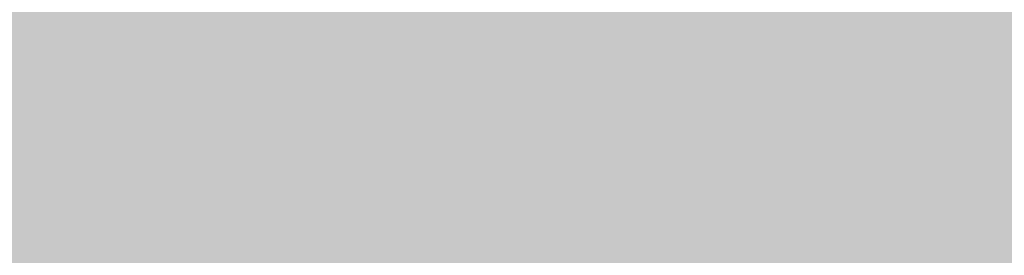
# Model space of a CAD drawing. Units: millimetres. Extents: x 0 to 2267, y 0 to 1823.
# Tile 200 of 256: x 1838.83 to 1841.442, y 1127.775 to 1128.399. Entities that reach past the tile are written whole.
import ezdxf

# ---------------------------------------------------------------- set-up
doc = ezdxf.new("R2010")
doc.units = ezdxf.units.MM
doc.header["$MEASUREMENT"] = 0
doc.layers.add('M-HATC', color=252, linetype='Continuous', lineweight=18)

msp = doc.modelspace()

# ---------------------------------------------------------------- hatches: boundary and pattern name
at = {"layer": 'M-HATC'}
h = msp.add_hatch(color=256, dxfattribs=at)
h.dxf.hatch_style = 1
h.paths.add_polyline_path([(2055.771, 1603.062), (1381.0868, 1603.062), (1381.0868, 1598.062), (2055.771, 1598.062)])
h.paths.add_polyline_path([(2055.771, 1598.062), (1381.0868, 1598.062), (1381.0868, 1593.062), (2055.771, 1593.062)])
h.paths.add_polyline_path([(2051.3074, 1536.7609), (1385.5504, 1536.7609), (1385.5504, 1526.7609), (1387.5504, 1526.7609), (1388.5366, 1525.0528), (1385.3319, 1521.2335), (1385.3319, 1521.2226), (2050.2542, 1522.7491), (2048.3212, 1525.0528), (2049.3074, 1526.7609), (2051.3074, 1526.7609)])
edge = h.paths.add_edge_path()
edge.add_arc((1847.5345, 1379.1492), 135, 222.603061, 222.890851, ccw=False)
edge.add_line((1748.1663, 1287.7656), (1683.0921, 1287.7656))
edge.add_arc((1583.7239, 1379.1492), 135, 317.109149, 317.396939, ccw=False)
edge.add_arc((1678.9686, 1290.6707), 5, 222.8909, 317.1091, ccw=False)
edge.add_arc((1774.2133, 1379.1492), 135, 222.603061, 222.890851, ccw=False)
edge.add_line((1674.8451, 1287.7656), (1609.7709, 1287.7656))
edge.add_arc((1510.4027, 1379.1492), 135, 317.109149, 317.396939, ccw=False)
edge.add_arc((1605.6474, 1290.6707), 5, 222.8909, 317.1091, ccw=False)
edge.add_arc((1700.8921, 1379.1492), 135, 222.603061, 222.890851, ccw=False)
edge.add_line((1601.5239, 1287.7656), (1536.4497, 1287.7656))
edge.add_arc((1437.0815, 1379.1492), 135, 317.109149, 317.396939, ccw=False)
edge.add_arc((1532.3262, 1290.6707), 5, 222.8909, 317.1091, ccw=False)
edge.add_arc((1627.5709, 1379.1492), 135, 222.603061, 222.890851, ccw=False)
edge.add_line((1528.2027, 1287.7656), (1505.9289, 1287.7656))
edge.add_spline(control_points=[(1505.9289, 1287.7656), (1504.2622, 1287.7656), (1504.2622, 1282.7656), (1505.9289, 1282.7656)], knot_values=[0, 0, 0, 0, 5, 5, 5, 5], degree=3, periodic=0)
edge.add_line((1505.9289, 1282.7656), (1930.9289, 1282.7656))
edge.add_spline(control_points=[(1930.9289, 1282.7656), (1932.5956, 1282.7656), (1932.5956, 1287.7656), (1930.9289, 1287.7656)], knot_values=[0, 0, 0, 0, 5, 5, 5, 5], degree=3, periodic=0)
edge.add_line((1930.9289, 1287.7656), (1903.0557, 1287.7656))
edge.add_arc((1803.6875, 1379.1492), 135, 317.109149, 317.396939, ccw=False)
edge.add_arc((1898.9322, 1290.6707), 5, 222.8909, 317.1091, ccw=False)
edge.add_arc((1994.1769, 1379.1492), 135, 222.603061, 222.890851, ccw=False)
edge.add_line((1894.8087, 1287.7656), (1829.7345, 1287.7656))
edge.add_arc((1730.3663, 1379.1492), 135, 317.109149, 317.396939, ccw=False)
edge.add_arc((1825.611, 1290.6707), 5, 222.8909, 317.1091, ccw=False)
edge.add_arc((1920.8557, 1379.1492), 135, 222.603061, 222.890851, ccw=False)
edge.add_line((1821.4875, 1287.7656), (1756.4133, 1287.7656))
edge.add_arc((1657.0451, 1379.1492), 135, 317.109149, 317.396939, ccw=False)
edge.add_arc((1752.2898, 1290.6707), 5, 222.8909, 317.1091, ccw=False)
edge = h.paths.add_edge_path()
edge.add_spline(control_points=[(1843.4289, 1227.2475), (1845.0956, 1227.2475), (1845.0956, 1232.2475), (1843.4289, 1232.2475)], knot_values=[0, 0, 0, 0, 5, 5, 5, 5], degree=3, periodic=0)
edge.add_line((1843.4289, 1232.2475), (1593.4289, 1232.2475))
edge.add_spline(control_points=[(1593.4289, 1232.2475), (1591.7622, 1232.2475), (1591.7622, 1227.2475), (1593.4289, 1227.2475)], knot_values=[0, 0, 0, 0, 5, 5, 5, 5], degree=3, periodic=0)
edge.add_line((1593.4289, 1227.2475), (1843.4289, 1227.2475))
h.paths.add_polyline_path([(1905.9289, 1127.4171), (1530.9289, 1127.4171, 0.414214), (1520.9289, 1117.4171), (1530.9289, 1117.4171), (1915.9289, 1117.4171, 0.414214)])
edge = h.paths.add_edge_path()
edge.add_arc((1397.0858, 1498.4078), 12.7299, 90.78215, 190.87871, ccw=False)
edge.add_line((1396.912, 1511.1365), (1428.0097, 1511.3488))
edge.add_line((1428.0097, 1511.3488), (1433.0097, 1511.3488))
edge.add_line((1433.0097, 1511.3488), (1434.439, 1511.3488))
edge.add_arc((1419.474, 1498.0804), 20, 41.561, 74.08211)
edge.add_line((1424.9592, 1517.3135), (1399.9351, 1517.2561))
edge.add_spline(control_points=[(1399.9307, 1517.2561), (1399.884, 1517.2131), (1399.8328, 1517.1689), (1399.7774, 1517.1236)], knot_values=[11.567499, 11.567499, 11.567499, 11.567499, 11.814249, 11.814249, 11.814249, 11.814249], degree=3, periodic=0)
edge.add_spline(control_points=[(1399.6328, 1517.0099), (1399.5831, 1516.9721), (1399.5307, 1516.9338), (1399.4759, 1516.8947)], knot_values=[11.167718, 11.167718, 11.167718, 11.167718, 11.365188, 11.365188, 11.365188, 11.365188], degree=3, periodic=0)
edge.add_spline(control_points=[(1399.3398, 1516.8001), (1399.1514, 1516.6719), (1398.9384, 1516.5377), (1398.704, 1516.3994)], knot_values=[10.376405, 10.376405, 10.376405, 10.376405, 11.00994, 11.00994, 11.00994, 11.00994], degree=3, periodic=0)
edge.add_spline(control_points=[(1398.6572, 1516.3719), (1398.5789, 1516.326), (1398.4983, 1516.2797), (1398.4155, 1516.2331)], knot_values=[10.125175, 10.125175, 10.125175, 10.125175, 10.334406, 10.334406, 10.334406, 10.334406], degree=3, periodic=0)
edge.add_spline(control_points=[(1398.2642, 1516.1487), (1398.196, 1516.1111), (1398.1263, 1516.0732), (1398.0555, 1516.0351)], knot_values=[9.832246, 9.832246, 9.832246, 9.832246, 9.999658, 9.999658, 9.999658, 9.999658], degree=3, periodic=0)
edge.add_spline(control_points=[(1397.9987, 1516.0048), (1397.7312, 1515.8621), (1397.446, 1515.7171), (1397.1466, 1515.5714)], knot_values=[9.161808, 9.161808, 9.161808, 9.161808, 9.787769, 9.787769, 9.787769, 9.787769], degree=3, periodic=0)
edge.add_spline(control_points=[(1397.1466, 1515.5714), (1396.8418, 1515.423), (1396.5222, 1515.274), (1396.1914, 1515.1262)], knot_values=[8.524455, 8.524455, 8.524455, 8.524455, 9.161808, 9.161808, 9.161808, 9.161808], degree=3, periodic=0)
edge.add_spline(control_points=[(1396.0777, 1515.0756), (1395.9854, 1515.0348), (1395.8922, 1514.994), (1395.7983, 1514.9534)], knot_values=[8.275193, 8.275193, 8.275193, 8.275193, 8.451726, 8.451726, 8.451726, 8.451726], degree=3, periodic=0)
edge.add_spline(control_points=[(1395.6018, 1514.8691), (1395.4997, 1514.8257), (1395.3968, 1514.7824), (1395.2932, 1514.7394)], knot_values=[7.962917, 7.962917, 7.962917, 7.962917, 8.152764, 8.152764, 8.152764, 8.152764], degree=3, periodic=0)
edge.add_spline(control_points=[(1395.2116, 1514.7057), (1394.8278, 1514.5475), (1394.4345, 1514.3929), (1394.0364, 1514.2442)], knot_values=[7.21254, 7.21254, 7.21254, 7.21254, 7.913148, 7.913148, 7.913148, 7.913148], degree=3, periodic=0)
edge.add_spline(control_points=[(1394.0364, 1514.2442), (1393.7076, 1514.1214), (1393.3754, 1514.0027), (1393.0427, 1513.8895)], knot_values=[6.633733, 6.633733, 6.633733, 6.633733, 7.21254, 7.21254, 7.21254, 7.21254], degree=3, periodic=0)
edge.add_spline(control_points=[(1392.8214, 1513.815), (1392.7198, 1513.7812), (1392.6181, 1513.7479), (1392.5166, 1513.7152)], knot_values=[6.328796, 6.328796, 6.328796, 6.328796, 6.505493, 6.505493, 6.505493, 6.505493], degree=3, periodic=0)
edge.add_spline(control_points=[(1392.5166, 1513.7152), (1392.3187, 1513.6515), (1392.1212, 1513.59), (1391.9244, 1513.531)], knot_values=[5.984605, 5.984605, 5.984605, 5.984605, 6.328796, 6.328796, 6.328796, 6.328796], degree=3, periodic=0)
edge.add_spline(control_points=[(1391.7915, 1513.4915), (1391.3122, 1513.3501), (1390.8384, 1513.2239), (1390.3784, 1513.1171)], knot_values=[5.066697, 5.066697, 5.066697, 5.066697, 5.907055, 5.907055, 5.907055, 5.907055], degree=3, periodic=0)
edge.add_spline(control_points=[(1390.3784, 1513.1171), (1390.1797, 1513.071), (1389.9836, 1513.0284), (1389.7907, 1512.9899)], knot_values=[4.70367, 4.70367, 4.70367, 4.70367, 5.066695, 5.066695, 5.066695, 5.066695], degree=3, periodic=0)
edge.add_spline(control_points=[(1389.422, 1512.9204), (1389.2459, 1512.8892), (1389.0729, 1512.8617), (1388.9036, 1512.8381)], knot_values=[4.130571, 4.130571, 4.130571, 4.130571, 4.469816, 4.469816, 4.469816, 4.469816], degree=3, periodic=0)
edge.add_spline(control_points=[(1388.9036, 1512.8381), (1388.591, 1512.7946), (1388.2911, 1512.7644), (1388.0071, 1512.7494)], knot_values=[3.504031, 3.504031, 3.504031, 3.504031, 4.130571, 4.130571, 4.130571, 4.130571], degree=3, periodic=0)
edge.add_spline(control_points=[(1387.9356, 1512.7459), (1387.8538, 1512.7423), (1387.7733, 1512.74), (1387.6944, 1512.739)], knot_values=[3.268866, 3.268866, 3.268866, 3.268866, 3.451164, 3.451164, 3.451164, 3.451164], degree=3, periodic=0)
edge.add_spline(control_points=[(1387.3351, 1512.7443), (1387.2076, 1512.7499), (1387.0847, 1512.7597), (1386.967, 1512.7739)], knot_values=[2.670686, 2.670686, 2.670686, 2.670686, 2.984, 2.984, 2.984, 2.984], degree=3, periodic=0)
edge.add_spline(control_points=[(1386.8327, 1512.7922), (1386.8209, 1512.7941), (1386.8092, 1512.7959), (1386.7975, 1512.7979)], knot_values=[2.516981, 2.516981, 2.516981, 2.516981, 2.549528, 2.549528, 2.549528, 2.549528], degree=3, periodic=0)
edge.add_spline(control_points=[(1386.4526, 1512.8735), (1386.4257, 1512.881), (1386.3993, 1512.889), (1386.3733, 1512.8972)], knot_values=[2.095869, 2.095869, 2.095869, 2.095869, 2.17941, 2.17941, 2.17941, 2.17941], degree=3, periodic=0)
edge.add_spline(control_points=[(1386.0691, 1513.0189), (1386.0634, 1513.0217), (1386.0577, 1513.0246), (1386.052, 1513.0275)], knot_values=[1.72453, 1.72453, 1.72453, 1.72453, 1.745933, 1.745933, 1.745933, 1.745933], degree=3, periodic=0)
edge.add_arc((1399.474, 1498.0804), 20, 131.82432, 180)
edge.add_arc((1630.3336, 1505.5484), 250.9708, 181.705176, 236.427975)
edge.add_arc((1605.3399, 1483.3044), 218.7822, 238.660829, 243.34961)
edge.add_arc((1647.0911, 1510.3592), 262.8986, 183.129836, 237.853442, ccw=False)
h.paths.add_polyline_path([(1406.5369, 1391.9644, 0.149382), (1491.5506, 1296.4418, -0.129517)], flags=17)
edge = h.paths.add_edge_path()
edge.add_arc((2037.3838, 1498.0804), 20, 0, 48.26587)
edge.add_spline(control_points=[(2050.6973, 1513.0052), (2050.6512, 1512.9847), (2050.6034, 1512.9655), (2050.5539, 1512.9477)], knot_values=[1.835652, 1.835652, 1.835652, 1.835652, 2.000781, 2.000781, 2.000781, 2.000781], degree=3, periodic=0)
edge.add_spline(control_points=[(2050.4616, 1512.9166), (2050.479, 1512.9221), (2050.4963, 1512.9277), (2050.5133, 1512.9335)], knot_values=[2.045477, 2.045477, 2.045477, 2.045477, 2.101389, 2.101389, 2.101389, 2.101389], degree=3, periodic=0)
edge.add_spline(control_points=[(2050.129, 1512.8342), (2050.1984, 1512.8473), (2050.2657, 1512.8623), (2050.3308, 1512.8792)], knot_values=[2.237629, 2.237629, 2.237629, 2.237629, 2.435841, 2.435841, 2.435841, 2.435841], degree=3, periodic=0)
edge.add_spline(control_points=[(2050.0946, 1512.8278), (2050.1061, 1512.8299), (2050.1176, 1512.832), (2050.129, 1512.8342)], knot_values=[2.435841, 2.435841, 2.435841, 2.435841, 2.468321, 2.468321, 2.468321, 2.468321], degree=3, periodic=0)
edge.add_spline(control_points=[(2049.7843, 1512.7851), (2049.8552, 1512.7922), (2049.9243, 1512.8008), (2049.9917, 1512.8109)], knot_values=[2.563852, 2.563852, 2.563852, 2.563852, 2.748541, 2.748541, 2.748541, 2.748541], degree=3, periodic=0)
edge.add_spline(control_points=[(2049.4052, 1512.7617), (2049.5364, 1512.7653), (2049.6629, 1512.773), (2049.7843, 1512.7851)], knot_values=[2.748541, 2.748541, 2.748541, 2.748541, 3.064882, 3.064882, 3.064882, 3.064882], degree=3, periodic=0)
edge.add_spline(control_points=[(2049.1698, 1512.7597), (2049.2336, 1512.7591), (2049.2965, 1512.7594), (2049.3584, 1512.7606)], knot_values=[3.102309, 3.102309, 3.102309, 3.102309, 3.2503, 3.2503, 3.2503, 3.2503], degree=3, periodic=0)
edge.add_spline(control_points=[(2048.8573, 1512.7691), (2048.9638, 1512.7638), (2049.068, 1512.7606), (2049.1698, 1512.7597)], knot_values=[3.2503, 3.2503, 3.2503, 3.2503, 3.486069, 3.486069, 3.486069, 3.486069], degree=3, periodic=0)
edge.add_spline(control_points=[(2048.6924, 1512.7789), (2048.3729, 1512.8009), (2048.0345, 1512.8411), (2047.6817, 1512.897)], knot_values=[3.606429, 3.606429, 3.606429, 3.606429, 4.2989, 4.2989, 4.2989, 4.2989], degree=3, periodic=0)
edge.add_spline(control_points=[(2047.6817, 1512.897), (2047.5458, 1512.9185), (2047.4077, 1512.9424), (2047.2678, 1512.9685)], knot_values=[4.2989, 4.2989, 4.2989, 4.2989, 4.565769, 4.565769, 4.565769, 4.565769], degree=3, periodic=0)
edge.add_spline(control_points=[(2047.2678, 1512.9685), (2047.1449, 1512.9914), (2047.0207, 1513.016), (2046.8951, 1513.0422)], knot_values=[4.565769, 4.565769, 4.565769, 4.565769, 4.799971, 4.799971, 4.799971, 4.799971], degree=3, periodic=0)
edge.add_spline(control_points=[(2046.8951, 1513.0422), (2046.5286, 1513.1188), (2046.1513, 1513.209), (2045.7676, 1513.3107)], knot_values=[4.799971, 4.799971, 4.799971, 4.799971, 5.483718, 5.483718, 5.483718, 5.483718], degree=3, periodic=0)
edge.add_spline(control_points=[(2045.7676, 1513.3107), (2045.3724, 1513.4154), (2044.9704, 1513.5322), (2044.5662, 1513.6588)], knot_values=[5.483718, 5.483718, 5.483718, 5.483718, 6.187866, 6.187866, 6.187866, 6.187866], degree=3, periodic=0)
edge.add_spline(control_points=[(2044.5662, 1513.6588), (2044.4149, 1513.7061), (2044.2633, 1513.7549), (2044.1116, 1513.8048)], knot_values=[6.187866, 6.187866, 6.187866, 6.187866, 6.451551, 6.451551, 6.451551, 6.451551], degree=3, periodic=0)
edge.add_spline(control_points=[(2044.1116, 1513.8048), (2043.9967, 1513.8427), (2043.8817, 1513.8813), (2043.7668, 1513.9205)], knot_values=[6.451551, 6.451551, 6.451551, 6.451551, 6.651434, 6.651434, 6.651434, 6.651434], degree=3, periodic=0)
edge.add_spline(control_points=[(2043.7668, 1513.9205), (2043.3716, 1514.0554), (2042.9774, 1514.1979), (2042.5886, 1514.3458)], knot_values=[6.651434, 6.651434, 6.651434, 6.651434, 7.338879, 7.338879, 7.338879, 7.338879], degree=3, periodic=0)
edge.add_spline(control_points=[(2042.5886, 1514.3458), (2042.1643, 1514.5071), (2041.7465, 1514.6749), (2041.3409, 1514.846)], knot_values=[7.338879, 7.338879, 7.338879, 7.338879, 8.089209, 8.089209, 8.089209, 8.089209], degree=3, periodic=0)
edge.add_spline(control_points=[(2041.3409, 1514.846), (2041.1028, 1514.9465), (2040.869, 1515.0481), (2040.6405, 1515.1502)], knot_values=[8.089209, 8.089209, 8.089209, 8.089209, 8.529587, 8.529587, 8.529587, 8.529587], degree=3, periodic=0)
edge.add_spline(control_points=[(2040.51, 1515.2089), (2040.0824, 1515.4022), (2039.6747, 1515.5971), (2039.295, 1515.7894)], knot_values=[8.613818, 8.613818, 8.613818, 8.613818, 9.44571, 9.44571, 9.44571, 9.44571], degree=3, periodic=0)
edge.add_spline(control_points=[(2039.295, 1515.7894), (2039.0618, 1515.9075), (2038.8391, 1516.0246), (2038.6288, 1516.1398)], knot_values=[9.44571, 9.44571, 9.44571, 9.44571, 9.956404, 9.956404, 9.956404, 9.956404], degree=3, periodic=0)
edge.add_spline(control_points=[(2038.6288, 1516.1398), (2038.5187, 1516.2001), (2038.4121, 1516.2598), (2038.309, 1516.3189)], knot_values=[9.956404, 9.956404, 9.956404, 9.956404, 10.223542, 10.223542, 10.223542, 10.223542], degree=3, periodic=0)
edge.add_spline(control_points=[(2038.309, 1516.3189), (2038.2138, 1516.3735), (2038.1216, 1516.4276), (2038.0328, 1516.481)], knot_values=[10.223542, 10.223542, 10.223542, 10.223542, 10.47051, 10.47051, 10.47051, 10.47051], degree=3, periodic=0)
edge.add_spline(control_points=[(2038.0328, 1516.481), (2037.7855, 1516.6296), (2037.5639, 1516.773), (2037.3722, 1516.909)], knot_values=[10.47051, 10.47051, 10.47051, 10.47051, 11.15767, 11.15767, 11.15767, 11.15767], degree=3, periodic=0)
edge.add_spline(control_points=[(2037.3722, 1516.909), (2037.2789, 1516.9752), (2037.1927, 1517.0396), (2037.1142, 1517.102)], knot_values=[11.15767, 11.15767, 11.15767, 11.15767, 11.49227, 11.49227, 11.49227, 11.49227], degree=3, periodic=0)
edge.add_spline(control_points=[(2036.8564, 1517.3259), (2036.9148, 1517.2692), (2036.9814, 1517.2103), (2037.0557, 1517.1492)], knot_values=[11.577341, 11.577341, 11.577341, 11.577341, 11.91035, 11.91035, 11.91035, 11.91035], degree=3, periodic=0)
edge.add_spline(control_points=[(2036.8074, 1517.3748), (2036.823, 1517.3587), (2036.8393, 1517.3424), (2036.8564, 1517.3259)], knot_values=[11.91035, 11.91035, 11.91035, 11.91035, 12.007402, 12.007402, 12.007402, 12.007402], degree=3, periodic=0)
edge.add_spline(control_points=[(2036.7017, 1517.494), (2036.7104, 1517.483), (2036.7196, 1517.4719), (2036.7291, 1517.4606)], knot_values=[12.184155, 12.184155, 12.184155, 12.184155, 12.255409, 12.255409, 12.255409, 12.255409], degree=3, periodic=0)
edge.add_spline(control_points=[(2036.6159, 1517.6205), (2036.62, 1517.613), (2036.6243, 1517.6055), (2036.6289, 1517.5979)], knot_values=[12.487913, 12.487913, 12.487913, 12.487913, 12.541035, 12.541035, 12.541035, 12.541035], degree=3, periodic=0)
edge.add_spline(control_points=[(2036.5635, 1517.786), (2036.5637, 1517.7794), (2036.5642, 1517.7726), (2036.565, 1517.7658)], knot_values=[12.911761, 12.911761, 12.911761, 12.911761, 12.968286, 12.968286, 12.968286, 12.968286], degree=3, periodic=0)
edge.add_spline(control_points=[(2036.6166, 1517.9304), (2036.6125, 1517.9259), (2036.6086, 1517.9212), (2036.6049, 1517.9165)], knot_values=[13.382527, 13.382527, 13.382527, 13.382527, 13.433791, 13.433791, 13.433791, 13.433791], degree=3, periodic=0)
edge.add_spline(control_points=[(2036.749, 1518.017), (2036.7361, 1518.0116), (2036.7239, 1518.006), (2036.7124, 1518.0002)], knot_values=[13.726299, 13.726299, 13.726299, 13.726299, 13.809928, 13.809928, 13.809928, 13.809928], degree=3, periodic=0)
edge.add_spline(control_points=[(2036.8604, 1518.0528), (2036.8386, 1518.0474), (2036.8181, 1518.0416), (2036.7988, 1518.0353)], knot_values=[13.910887, 13.910887, 13.910887, 13.910887, 14.02153, 14.02153, 14.02153, 14.02153], degree=3, periodic=0)
edge.add_line((2036.9639, 1518.0804), (2032.3838, 1518.0804))
edge.add_line((2032.3838, 1518.0804), (2027.3838, 1518.0804))
edge.add_line((2027.3838, 1518.0804), (2022.3838, 1518.0804))
edge.add_line((2022.3838, 1518.0804), (2017.3838, 1518.0804))
edge.add_arc((2017.3838, 1498.0804), 20, 90, 138.439)
edge.add_line((2002.4188, 1511.3488), (2003.8481, 1511.3488))
edge.add_line((2003.8481, 1511.3488), (2008.8481, 1511.3488))
edge.add_line((2008.8481, 1511.3488), (2039.772, 1511.1377))
edge.add_arc((2039.772, 1498.4078), 12.7299, -10.87871, 90, ccw=False)
edge.add_arc((1789.7668, 1510.3592), 262.8986, 302.146558, 356.870164, ccw=False)
edge.add_arc((1831.5179, 1483.3044), 218.7822, 296.65039, 301.339171)
edge.add_arc((1806.5242, 1505.5484), 250.9708, 303.572025, 358.294824)
h.paths.add_polyline_path([(2030.321, 1391.9644, -0.129517), (1945.3072, 1296.4418, 0.149382)], flags=17)
edge = h.paths.add_edge_path()
edge.add_spline(control_points=[(2037.2464, 1518.0821), (2037.2898, 1518.081), (2037.3355, 1518.0804), (2037.3838, 1518.0804)], knot_values=[0.000012, 0.000012, 0.000012, 0.000012, 0.144754, 0.144754, 0.144754, 0.144754], degree=3, periodic=0)
edge.add_line((2037.3357, 1518.0804), (2037.0096, 1518.0804))
edge.add_spline(control_points=[(2037.0096, 1518.0804), (2036.9822, 1518.0768), (2036.956, 1518.0727), (2036.9312, 1518.0681)], knot_values=[14.13465, 14.13465, 14.13465, 14.13465, 14.247197, 14.247197, 14.247197, 14.247197], degree=3, periodic=0)
edge.add_spline(control_points=[(2036.9312, 1518.0681), (2036.9276, 1518.0674), (2036.9241, 1518.0667), (2036.9205, 1518.0661)], knot_values=[14.118315, 14.118315, 14.118315, 14.118315, 14.13465, 14.13465, 14.13465, 14.13465], degree=3, periodic=0)
edge.add_spline(control_points=[(2036.9205, 1518.0661), (2036.9118, 1518.0644), (2036.9032, 1518.0626), (2036.8948, 1518.0608)], knot_values=[14.078086, 14.078086, 14.078086, 14.078086, 14.118315, 14.118315, 14.118315, 14.118315], degree=3, periodic=0)
edge.add_spline(control_points=[(2036.8948, 1518.0608), (2036.883, 1518.0583), (2036.8716, 1518.0556), (2036.8604, 1518.0528)], knot_values=[14.02153, 14.02153, 14.02153, 14.02153, 14.078086, 14.078086, 14.078086, 14.078086], degree=3, periodic=0)
edge.add_spline(control_points=[(2036.8604, 1518.0528), (2036.8386, 1518.0474), (2036.8181, 1518.0416), (2036.7988, 1518.0353)], knot_values=[13.910887, 13.910887, 13.910887, 13.910887, 14.02153, 14.02153, 14.02153, 14.02153], degree=3, periodic=0)
edge.add_spline(control_points=[(2036.7988, 1518.0353), (2036.7981, 1518.035), (2036.7974, 1518.0348), (2036.7967, 1518.0346)], knot_values=[13.906906, 13.906906, 13.906906, 13.906906, 13.910887, 13.910887, 13.910887, 13.910887], degree=3, periodic=0)
edge.add_spline(control_points=[(2036.7967, 1518.0346), (2036.7882, 1518.0318), (2036.7799, 1518.0289), (2036.7719, 1518.0259)], knot_values=[13.857826, 13.857826, 13.857826, 13.857826, 13.906906, 13.906906, 13.906906, 13.906906], degree=3, periodic=0)
edge.add_spline(control_points=[(2036.7719, 1518.0259), (2036.764, 1518.023), (2036.7564, 1518.02), (2036.749, 1518.017)], knot_values=[13.809928, 13.809928, 13.809928, 13.809928, 13.857826, 13.857826, 13.857826, 13.857826], degree=3, periodic=0)
edge.add_spline(control_points=[(2036.749, 1518.017), (2036.7361, 1518.0116), (2036.7239, 1518.006), (2036.7124, 1518.0002)], knot_values=[13.726299, 13.726299, 13.726299, 13.726299, 13.809928, 13.809928, 13.809928, 13.809928], degree=3, periodic=0)
edge.add_spline(control_points=[(2036.7124, 1518.0002), (2036.7121, 1518), (2036.7118, 1517.9999), (2036.7115, 1517.9997)], knot_values=[13.723993, 13.723993, 13.723993, 13.723993, 13.726299, 13.726299, 13.726299, 13.726299], degree=3, periodic=0)
edge.add_spline(control_points=[(2036.7115, 1517.9997), (2036.7063, 1517.9971), (2036.7013, 1517.9944), (2036.6965, 1517.9917)], knot_values=[13.686536, 13.686536, 13.686536, 13.686536, 13.723993, 13.723993, 13.723993, 13.723993], degree=3, periodic=0)
edge.add_spline(control_points=[(2036.6965, 1517.9917), (2036.6919, 1517.9891), (2036.6874, 1517.9865), (2036.6831, 1517.9839)], knot_values=[13.651251, 13.651251, 13.651251, 13.651251, 13.686536, 13.686536, 13.686536, 13.686536], degree=3, periodic=0)
edge.add_spline(control_points=[(2036.6831, 1517.9839), (2036.6764, 1517.9798), (2036.67, 1517.9757), (2036.6639, 1517.9714)], knot_values=[13.596804, 13.596804, 13.596804, 13.596804, 13.651251, 13.651251, 13.651251, 13.651251], degree=3, periodic=0)
edge.add_spline(control_points=[(2036.6639, 1517.9714), (2036.6636, 1517.9712), (2036.6633, 1517.9709), (2036.6629, 1517.9707)], knot_values=[13.593956, 13.593956, 13.593956, 13.593956, 13.596804, 13.596804, 13.596804, 13.596804], degree=3, periodic=0)
edge.add_spline(control_points=[(2036.6629, 1517.9707), (2036.6603, 1517.9689), (2036.6577, 1517.967), (2036.6552, 1517.9651)], knot_values=[13.570322, 13.570322, 13.570322, 13.570322, 13.593956, 13.593956, 13.593956, 13.593956], degree=3, periodic=0)
edge.add_spline(control_points=[(2036.6552, 1517.9651), (2036.6525, 1517.9631), (2036.6499, 1517.9611), (2036.6474, 1517.9591)], knot_values=[13.545477, 13.545477, 13.545477, 13.545477, 13.570322, 13.570322, 13.570322, 13.570322], degree=3, periodic=0)
edge.add_spline(control_points=[(2036.6474, 1517.9591), (2036.6472, 1517.9589), (2036.6471, 1517.9588), (2036.6469, 1517.9587)], knot_values=[13.543931, 13.543931, 13.543931, 13.543931, 13.545477, 13.545477, 13.545477, 13.545477], degree=3, periodic=0)
edge.add_spline(control_points=[(2036.6469, 1517.9587), (2036.6412, 1517.9541), (2036.6358, 1517.9494), (2036.6307, 1517.9447)], knot_values=[13.488237, 13.488237, 13.488237, 13.488237, 13.543931, 13.543931, 13.543931, 13.543931], degree=3, periodic=0)
edge.add_spline(control_points=[(2036.6307, 1517.9447), (2036.6282, 1517.9423), (2036.6257, 1517.9399), (2036.6233, 1517.9374)], knot_values=[13.460307, 13.460307, 13.460307, 13.460307, 13.488237, 13.488237, 13.488237, 13.488237], degree=3, periodic=0)
edge.add_spline(control_points=[(2036.6233, 1517.9374), (2036.6215, 1517.9356), (2036.6198, 1517.9338), (2036.6181, 1517.932)], knot_values=[13.439712, 13.439712, 13.439712, 13.439712, 13.460307, 13.460307, 13.460307, 13.460307], degree=3, periodic=0)
edge.add_spline(control_points=[(2036.6181, 1517.932), (2036.6176, 1517.9315), (2036.6171, 1517.9309), (2036.6166, 1517.9304)], knot_values=[13.433791, 13.433791, 13.433791, 13.433791, 13.439712, 13.439712, 13.439712, 13.439712], degree=3, periodic=0)
edge.add_spline(control_points=[(2036.6166, 1517.9304), (2036.6125, 1517.9259), (2036.6086, 1517.9212), (2036.6049, 1517.9165)], knot_values=[13.382527, 13.382527, 13.382527, 13.382527, 13.433791, 13.433791, 13.433791, 13.433791], degree=3, periodic=0)
edge.add_spline(control_points=[(2036.6049, 1517.9165), (2036.6026, 1517.9135), (2036.6004, 1517.9104), (2036.5982, 1517.9074)], knot_values=[13.350017, 13.350017, 13.350017, 13.350017, 13.382527, 13.382527, 13.382527, 13.382527], degree=3, periodic=0)
edge.add_spline(control_points=[(2036.5982, 1517.9074), (2036.5972, 1517.9059), (2036.5962, 1517.9043), (2036.5952, 1517.9028)], knot_values=[13.333922, 13.333922, 13.333922, 13.333922, 13.350017, 13.350017, 13.350017, 13.350017], degree=3, periodic=0)
edge.add_spline(control_points=[(2036.5952, 1517.9028), (2036.5945, 1517.9018), (2036.5939, 1517.9009), (2036.5933, 1517.8999)], knot_values=[13.323828, 13.323828, 13.323828, 13.323828, 13.333922, 13.333922, 13.333922, 13.333922], degree=3, periodic=0)
edge.add_spline(control_points=[(2036.5933, 1517.8999), (2036.5905, 1517.8955), (2036.5879, 1517.8909), (2036.5855, 1517.8864)], knot_values=[13.277545, 13.277545, 13.277545, 13.277545, 13.323828, 13.323828, 13.323828, 13.323828], degree=3, periodic=0)
edge.add_spline(control_points=[(2036.5855, 1517.8864), (2036.5836, 1517.8827), (2036.5817, 1517.8789), (2036.5801, 1517.8751)], knot_values=[13.240119, 13.240119, 13.240119, 13.240119, 13.277545, 13.277545, 13.277545, 13.277545], degree=3, periodic=0)
edge.add_spline(control_points=[(2036.5801, 1517.8751), (2036.5795, 1517.8739), (2036.579, 1517.8727), (2036.5785, 1517.8715)], knot_values=[13.228211, 13.228211, 13.228211, 13.228211, 13.240119, 13.240119, 13.240119, 13.240119], degree=3, periodic=0)
edge.add_spline(control_points=[(2036.5785, 1517.8715), (2036.578, 1517.8702), (2036.5774, 1517.869), (2036.5769, 1517.8677)], knot_values=[13.215717, 13.215717, 13.215717, 13.215717, 13.228211, 13.228211, 13.228211, 13.228211], degree=3, periodic=0)
edge.add_spline(control_points=[(2036.5769, 1517.8677), (2036.5755, 1517.864), (2036.5741, 1517.8603), (2036.5729, 1517.8565)], knot_values=[13.179847, 13.179847, 13.179847, 13.179847, 13.215717, 13.215717, 13.215717, 13.215717], degree=3, periodic=0)
edge.add_spline(control_points=[(2036.5729, 1517.8565), (2036.5713, 1517.8515), (2036.5699, 1517.8464), (2036.5687, 1517.8413)], knot_values=[13.132017, 13.132017, 13.132017, 13.132017, 13.179847, 13.179847, 13.179847, 13.179847], degree=3, periodic=0)
edge.add_spline(control_points=[(2036.5687, 1517.8413), (2036.5684, 1517.8402), (2036.5682, 1517.8392), (2036.568, 1517.8382)], knot_values=[13.122482, 13.122482, 13.122482, 13.122482, 13.132017, 13.132017, 13.132017, 13.132017], degree=3, periodic=0)
edge.add_spline(control_points=[(2036.568, 1517.8382), (2036.5676, 1517.8363), (2036.5672, 1517.8345), (2036.5669, 1517.8327)], knot_values=[13.105592, 13.105592, 13.105592, 13.105592, 13.122482, 13.122482, 13.122482, 13.122482], degree=3, periodic=0)
edge.add_spline(control_points=[(2036.5669, 1517.8327), (2036.5662, 1517.8292), (2036.5657, 1517.8257), (2036.5652, 1517.8222)], knot_values=[13.074063, 13.074063, 13.074063, 13.074063, 13.105592, 13.105592, 13.105592, 13.105592], degree=3, periodic=0)
edge.add_spline(control_points=[(2036.5652, 1517.8222), (2036.5652, 1517.8222), (2036.5652, 1517.8222), (2036.5652, 1517.8222)], knot_values=[13.074043, 13.074043, 13.074043, 13.074043, 13.074063, 13.074063, 13.074063, 13.074063], degree=3, periodic=0)
edge.add_spline(control_points=[(2036.5652, 1517.8222), (2036.5644, 1517.8164), (2036.5639, 1517.8106), (2036.5636, 1517.8046)], knot_values=[13.021884, 13.021884, 13.021884, 13.021884, 13.074043, 13.074043, 13.074043, 13.074043], degree=3, periodic=0)
edge.add_spline(control_points=[(2036.5636, 1517.8046), (2036.5636, 1517.804), (2036.5636, 1517.8034), (2036.5635, 1517.8028)], knot_values=[13.01674, 13.01674, 13.01674, 13.01674, 13.021884, 13.021884, 13.021884, 13.021884], degree=3, periodic=0)
edge.add_spline(control_points=[(2036.5635, 1517.8028), (2036.5634, 1517.8005), (2036.5634, 1517.7982), (2036.5634, 1517.7958)], knot_values=[12.996438, 12.996438, 12.996438, 12.996438, 13.01674, 13.01674, 13.01674, 13.01674], degree=3, periodic=0)
edge.add_spline(control_points=[(2036.5634, 1517.7958), (2036.5633, 1517.7926), (2036.5634, 1517.7893), (2036.5635, 1517.786)], knot_values=[12.968286, 12.968286, 12.968286, 12.968286, 12.996438, 12.996438, 12.996438, 12.996438], degree=3, periodic=0)
edge.add_spline(control_points=[(2036.5635, 1517.786), (2036.5637, 1517.7794), (2036.5642, 1517.7726), (2036.565, 1517.7658)], knot_values=[12.911761, 12.911761, 12.911761, 12.911761, 12.968286, 12.968286, 12.968286, 12.968286], degree=3, periodic=0)
edge.add_spline(control_points=[(2036.565, 1517.7658), (2036.565, 1517.7657), (2036.565, 1517.7656), (2036.565, 1517.7656)], knot_values=[12.911017, 12.911017, 12.911017, 12.911017, 12.911761, 12.911761, 12.911761, 12.911761], degree=3, periodic=0)
edge.add_spline(control_points=[(2036.565, 1517.7656), (2036.5654, 1517.7625), (2036.5658, 1517.7593), (2036.5663, 1517.7562)], knot_values=[12.88528, 12.88528, 12.88528, 12.88528, 12.911017, 12.911017, 12.911017, 12.911017], degree=3, periodic=0)
edge.add_spline(control_points=[(2036.5663, 1517.7562), (2036.5667, 1517.7534), (2036.5672, 1517.7506), (2036.5677, 1517.7478)], knot_values=[12.862519, 12.862519, 12.862519, 12.862519, 12.88528, 12.88528, 12.88528, 12.88528], degree=3, periodic=0)
edge.add_spline(control_points=[(2036.5677, 1517.7478), (2036.5678, 1517.7474), (2036.5679, 1517.7469), (2036.568, 1517.7465)], knot_values=[12.858885, 12.858885, 12.858885, 12.858885, 12.862519, 12.862519, 12.862519, 12.862519], degree=3, periodic=0)
edge.add_spline(control_points=[(2036.568, 1517.7465), (2036.5692, 1517.7399), (2036.5707, 1517.7332), (2036.5724, 1517.7264)], knot_values=[12.8053, 12.8053, 12.8053, 12.8053, 12.858885, 12.858885, 12.858885, 12.858885], degree=3, periodic=0)
edge.add_spline(control_points=[(2036.5724, 1517.7264), (2036.5734, 1517.7226), (2036.5745, 1517.7187), (2036.5756, 1517.7149)], knot_values=[12.775176, 12.775176, 12.775176, 12.775176, 12.8053, 12.8053, 12.8053, 12.8053], degree=3, periodic=0)
edge.add_spline(control_points=[(2036.5756, 1517.7149), (2036.5763, 1517.7125), (2036.577, 1517.7102), (2036.5778, 1517.7078)], knot_values=[12.756759, 12.756759, 12.756759, 12.756759, 12.775176, 12.775176, 12.775176, 12.775176], degree=3, periodic=0)
edge.add_spline(control_points=[(2036.5778, 1517.7078), (2036.5781, 1517.7067), (2036.5784, 1517.7057), (2036.5787, 1517.7047)], knot_values=[12.748742, 12.748742, 12.748742, 12.748742, 12.756759, 12.756759, 12.756759, 12.756759], degree=3, periodic=0)
edge.add_spline(control_points=[(2036.5787, 1517.7047), (2036.5808, 1517.6983), (2036.5831, 1517.6919), (2036.5856, 1517.6854)], knot_values=[12.69959, 12.69959, 12.69959, 12.69959, 12.748742, 12.748742, 12.748742, 12.748742], degree=3, periodic=0)
edge.add_spline(control_points=[(2036.5856, 1517.6854), (2036.5876, 1517.68), (2036.5898, 1517.6746), (2036.5921, 1517.6692)], knot_values=[12.659038, 12.659038, 12.659038, 12.659038, 12.69959, 12.69959, 12.69959, 12.69959], degree=3, periodic=0)
edge.add_spline(control_points=[(2036.5921, 1517.6692), (2036.594, 1517.6648), (2036.5959, 1517.6605), (2036.5979, 1517.6561)], knot_values=[12.626806, 12.626806, 12.626806, 12.626806, 12.659038, 12.659038, 12.659038, 12.659038], degree=3, periodic=0)
edge.add_spline(control_points=[(2036.5979, 1517.6561), (2036.5984, 1517.6551), (2036.5989, 1517.6541), (2036.5993, 1517.6531)], knot_values=[12.619394, 12.619394, 12.619394, 12.619394, 12.626806, 12.626806, 12.626806, 12.626806], degree=3, periodic=0)
edge.add_spline(control_points=[(2036.5993, 1517.6531), (2036.6043, 1517.6424), (2036.6099, 1517.6315), (2036.6159, 1517.6205)], knot_values=[12.541039, 12.541039, 12.541039, 12.541039, 12.619394, 12.619394, 12.619394, 12.619394], degree=3, periodic=0)
edge.add_spline(control_points=[(2036.6159, 1517.6205), (2036.6159, 1517.6205), (2036.6159, 1517.6205), (2036.6159, 1517.6205)], knot_values=[12.541035, 12.541035, 12.541035, 12.541035, 12.541039, 12.541039, 12.541039, 12.541039], degree=3, periodic=0)
edge.add_spline(control_points=[(2036.6159, 1517.6205), (2036.62, 1517.613), (2036.6243, 1517.6055), (2036.6289, 1517.5979)], knot_values=[12.487913, 12.487913, 12.487913, 12.487913, 12.541035, 12.541035, 12.541035, 12.541035], degree=3, periodic=0)
edge.add_spline(control_points=[(2036.6289, 1517.5979), (2036.6326, 1517.5916), (2036.6365, 1517.5853), (2036.6406, 1517.5789)], knot_values=[12.443982, 12.443982, 12.443982, 12.443982, 12.487913, 12.487913, 12.487913, 12.487913], degree=3, periodic=0)
edge.add_spline(control_points=[(2036.6406, 1517.5789), (2036.6414, 1517.5776), (2036.6423, 1517.5763), (2036.6431, 1517.5749)], knot_values=[12.434996, 12.434996, 12.434996, 12.434996, 12.443982, 12.443982, 12.443982, 12.443982], degree=3, periodic=0)
edge.add_spline(control_points=[(2036.6431, 1517.5749), (2036.6531, 1517.5596), (2036.6639, 1517.5439), (2036.6756, 1517.528)], knot_values=[12.329647, 12.329647, 12.329647, 12.329647, 12.434996, 12.434996, 12.434996, 12.434996], degree=3, periodic=0)
edge.add_spline(control_points=[(2036.6756, 1517.528), (2036.6839, 1517.5168), (2036.6925, 1517.5055), (2036.7017, 1517.494)], knot_values=[12.255409, 12.255409, 12.255409, 12.255409, 12.329647, 12.329647, 12.329647, 12.329647], degree=3, periodic=0)
edge.add_spline(control_points=[(2036.7017, 1517.494), (2036.7104, 1517.483), (2036.7196, 1517.4719), (2036.7291, 1517.4606)], knot_values=[12.184155, 12.184155, 12.184155, 12.184155, 12.255409, 12.255409, 12.255409, 12.255409], degree=3, periodic=0)
edge.add_spline(control_points=[(2036.7291, 1517.4606), (2036.7436, 1517.4435), (2036.759, 1517.4262), (2036.7753, 1517.4085)], knot_values=[12.075961, 12.075961, 12.075961, 12.075961, 12.184155, 12.184155, 12.184155, 12.184155], degree=3, periodic=0)
edge.add_spline(control_points=[(2036.7753, 1517.4085), (2036.7763, 1517.4075), (2036.7773, 1517.4064), (2036.7783, 1517.4054)], knot_values=[12.069502, 12.069502, 12.069502, 12.069502, 12.075961, 12.075961, 12.075961, 12.075961], degree=3, periodic=0)
edge.add_spline(control_points=[(2036.7783, 1517.4054), (2036.7877, 1517.3953), (2036.7974, 1517.385), (2036.8074, 1517.3748)], knot_values=[12.007402, 12.007402, 12.007402, 12.007402, 12.069502, 12.069502, 12.069502, 12.069502], degree=3, periodic=0)
edge.add_spline(control_points=[(2036.8074, 1517.3748), (2036.823, 1517.3587), (2036.8393, 1517.3424), (2036.8564, 1517.3259)], knot_values=[11.91035, 11.91035, 11.91035, 11.91035, 12.007402, 12.007402, 12.007402, 12.007402], degree=3, periodic=0)
edge.add_spline(control_points=[(2036.8564, 1517.3259), (2036.9148, 1517.2692), (2036.9814, 1517.2103), (2037.0557, 1517.1492)], knot_values=[11.577341, 11.577341, 11.577341, 11.577341, 11.91035, 11.91035, 11.91035, 11.91035], degree=3, periodic=0)
edge.add_spline(control_points=[(2037.0557, 1517.1492), (2037.0747, 1517.1336), (2037.0942, 1517.1179), (2037.1142, 1517.102)], knot_values=[11.49227, 11.49227, 11.49227, 11.49227, 11.577341, 11.577341, 11.577341, 11.577341], degree=3, periodic=0)
edge.add_spline(control_points=[(2037.1142, 1517.102), (2037.1927, 1517.0396), (2037.2789, 1516.9752), (2037.3722, 1516.909)], knot_values=[11.15767, 11.15767, 11.15767, 11.15767, 11.49227, 11.49227, 11.49227, 11.49227], degree=3, periodic=0)
edge.add_spline(control_points=[(2037.3722, 1516.909), (2037.5639, 1516.773), (2037.7855, 1516.6296), (2038.0328, 1516.481)], knot_values=[10.47051, 10.47051, 10.47051, 10.47051, 11.15767, 11.15767, 11.15767, 11.15767], degree=3, periodic=0)
edge.add_spline(control_points=[(2038.0328, 1516.481), (2038.1216, 1516.4276), (2038.2138, 1516.3735), (2038.309, 1516.3189)], knot_values=[10.223542, 10.223542, 10.223542, 10.223542, 10.47051, 10.47051, 10.47051, 10.47051], degree=3, periodic=0)
edge.add_spline(control_points=[(2038.309, 1516.3189), (2038.4121, 1516.2598), (2038.5187, 1516.2001), (2038.6288, 1516.1398)], knot_values=[9.956404, 9.956404, 9.956404, 9.956404, 10.223542, 10.223542, 10.223542, 10.223542], degree=3, periodic=0)
edge.add_spline(control_points=[(2038.6288, 1516.1398), (2038.8391, 1516.0246), (2039.0618, 1515.9075), (2039.295, 1515.7894)], knot_values=[9.44571, 9.44571, 9.44571, 9.44571, 9.956404, 9.956404, 9.956404, 9.956404], degree=3, periodic=0)
edge.add_spline(control_points=[(2039.295, 1515.7894), (2039.6747, 1515.5971), (2040.0824, 1515.4022), (2040.51, 1515.2089)], knot_values=[8.613818, 8.613818, 8.613818, 8.613818, 9.44571, 9.44571, 9.44571, 9.44571], degree=3, periodic=0)
edge.add_spline(control_points=[(2040.51, 1515.2089), (2040.5533, 1515.1893), (2040.5968, 1515.1697), (2040.6405, 1515.1502)], knot_values=[8.529587, 8.529587, 8.529587, 8.529587, 8.613818, 8.613818, 8.613818, 8.613818], degree=3, periodic=0)
edge.add_spline(control_points=[(2040.6405, 1515.1502), (2040.869, 1515.0481), (2041.1028, 1514.9465), (2041.3409, 1514.846)], knot_values=[8.089209, 8.089209, 8.089209, 8.089209, 8.529587, 8.529587, 8.529587, 8.529587], degree=3, periodic=0)
edge.add_spline(control_points=[(2041.3409, 1514.846), (2041.7465, 1514.6749), (2042.1643, 1514.5071), (2042.5886, 1514.3458)], knot_values=[7.338879, 7.338879, 7.338879, 7.338879, 8.089209, 8.089209, 8.089209, 8.089209], degree=3, periodic=0)
edge.add_spline(control_points=[(2042.5886, 1514.3458), (2042.9774, 1514.1979), (2043.3716, 1514.0554), (2043.7668, 1513.9205)], knot_values=[6.651434, 6.651434, 6.651434, 6.651434, 7.338879, 7.338879, 7.338879, 7.338879], degree=3, periodic=0)
edge.add_spline(control_points=[(2043.7668, 1513.9205), (2043.8817, 1513.8813), (2043.9967, 1513.8427), (2044.1116, 1513.8048)], knot_values=[6.451551, 6.451551, 6.451551, 6.451551, 6.651434, 6.651434, 6.651434, 6.651434], degree=3, periodic=0)
edge.add_spline(control_points=[(2044.1116, 1513.8048), (2044.2633, 1513.7549), (2044.4149, 1513.7061), (2044.5662, 1513.6588)], knot_values=[6.187866, 6.187866, 6.187866, 6.187866, 6.451551, 6.451551, 6.451551, 6.451551], degree=3, periodic=0)
edge.add_spline(control_points=[(2044.5662, 1513.6588), (2044.9704, 1513.5322), (2045.3724, 1513.4154), (2045.7676, 1513.3107)], knot_values=[5.483718, 5.483718, 5.483718, 5.483718, 6.187866, 6.187866, 6.187866, 6.187866], degree=3, periodic=0)
edge.add_spline(control_points=[(2045.7676, 1513.3107), (2046.1513, 1513.209), (2046.5286, 1513.1188), (2046.8951, 1513.0422)], knot_values=[4.799971, 4.799971, 4.799971, 4.799971, 5.483718, 5.483718, 5.483718, 5.483718], degree=3, periodic=0)
edge.add_spline(control_points=[(2046.8951, 1513.0422), (2047.0207, 1513.016), (2047.1449, 1512.9914), (2047.2678, 1512.9685)], knot_values=[4.565769, 4.565769, 4.565769, 4.565769, 4.799971, 4.799971, 4.799971, 4.799971], degree=3, periodic=0)
edge.add_spline(control_points=[(2047.2678, 1512.9685), (2047.4077, 1512.9424), (2047.5458, 1512.9185), (2047.6817, 1512.897)], knot_values=[4.2989, 4.2989, 4.2989, 4.2989, 4.565769, 4.565769, 4.565769, 4.565769], degree=3, periodic=0)
edge.add_spline(control_points=[(2047.6817, 1512.897), (2048.0345, 1512.8411), (2048.3729, 1512.8009), (2048.6924, 1512.7789)], knot_values=[3.606429, 3.606429, 3.606429, 3.606429, 4.2989, 4.2989, 4.2989, 4.2989], degree=3, periodic=0)
edge.add_spline(control_points=[(2048.6924, 1512.7789), (2048.7479, 1512.7751), (2048.8029, 1512.7718), (2048.8573, 1512.7691)], knot_values=[3.486069, 3.486069, 3.486069, 3.486069, 3.606429, 3.606429, 3.606429, 3.606429], degree=3, periodic=0)
edge.add_spline(control_points=[(2048.8573, 1512.7691), (2048.9638, 1512.7638), (2049.068, 1512.7606), (2049.1698, 1512.7597)], knot_values=[3.2503, 3.2503, 3.2503, 3.2503, 3.486069, 3.486069, 3.486069, 3.486069], degree=3, periodic=0)
edge.add_spline(control_points=[(2049.1698, 1512.7597), (2049.2336, 1512.7591), (2049.2965, 1512.7594), (2049.3584, 1512.7606)], knot_values=[3.102309, 3.102309, 3.102309, 3.102309, 3.2503, 3.2503, 3.2503, 3.2503], degree=3, periodic=0)
edge.add_spline(control_points=[(2049.3584, 1512.7606), (2049.3741, 1512.7609), (2049.3897, 1512.7613), (2049.4052, 1512.7617)], knot_values=[3.064882, 3.064882, 3.064882, 3.064882, 3.102309, 3.102309, 3.102309, 3.102309], degree=3, periodic=0)
edge.add_spline(control_points=[(2049.4052, 1512.7617), (2049.5364, 1512.7653), (2049.6629, 1512.773), (2049.7843, 1512.7851)], knot_values=[2.748541, 2.748541, 2.748541, 2.748541, 3.064882, 3.064882, 3.064882, 3.064882], degree=3, periodic=0)
edge.add_spline(control_points=[(2049.7843, 1512.7851), (2049.8552, 1512.7922), (2049.9243, 1512.8008), (2049.9917, 1512.8109)], knot_values=[2.563852, 2.563852, 2.563852, 2.563852, 2.748541, 2.748541, 2.748541, 2.748541], degree=3, periodic=0)
edge.add_spline(control_points=[(2049.9917, 1512.8109), (2050.0265, 1512.8161), (2050.0608, 1512.8218), (2050.0946, 1512.8278)], knot_values=[2.468321, 2.468321, 2.468321, 2.468321, 2.563852, 2.563852, 2.563852, 2.563852], degree=3, periodic=0)
edge.add_spline(control_points=[(2050.0946, 1512.8278), (2050.1061, 1512.8299), (2050.1176, 1512.832), (2050.129, 1512.8342)], knot_values=[2.435841, 2.435841, 2.435841, 2.435841, 2.468321, 2.468321, 2.468321, 2.468321], degree=3, periodic=0)
edge.add_spline(control_points=[(2050.129, 1512.8342), (2050.1984, 1512.8473), (2050.2657, 1512.8623), (2050.3308, 1512.8792)], knot_values=[2.237629, 2.237629, 2.237629, 2.237629, 2.435841, 2.435841, 2.435841, 2.435841], degree=3, periodic=0)
edge.add_spline(control_points=[(2050.3308, 1512.8792), (2050.3754, 1512.8908), (2050.4191, 1512.9032), (2050.4616, 1512.9166)], knot_values=[2.101389, 2.101389, 2.101389, 2.101389, 2.237629, 2.237629, 2.237629, 2.237629], degree=3, periodic=0)
edge.add_spline(control_points=[(2050.4616, 1512.9166), (2050.479, 1512.9221), (2050.4963, 1512.9277), (2050.5133, 1512.9335)], knot_values=[2.045477, 2.045477, 2.045477, 2.045477, 2.101389, 2.101389, 2.101389, 2.101389], degree=3, periodic=0)
edge.add_spline(control_points=[(2050.5133, 1512.9335), (2050.527, 1512.9382), (2050.5405, 1512.9429), (2050.5539, 1512.9477)], knot_values=[2.000781, 2.000781, 2.000781, 2.000781, 2.045477, 2.045477, 2.045477, 2.045477], degree=3, periodic=0)
edge.add_spline(control_points=[(2050.5539, 1512.9477), (2050.6034, 1512.9655), (2050.6512, 1512.9847), (2050.6973, 1513.0052)], knot_values=[1.835652, 1.835652, 1.835652, 1.835652, 2.000781, 2.000781, 2.000781, 2.000781], degree=3, periodic=0)
edge.add_arc((2037.3838, 1498.0804), 20, 48.26587, 90.12993)
edge = h.paths.add_edge_path(flags=16)
edge.add_spline(control_points=[(1386.1389, 1512.9859), (1388.92, 1511.7395), (1398.0387, 1515.5187), (1399.9307, 1517.2561)], knot_values=[1.831046, 1.831046, 1.831046, 1.831046, 11.814249, 11.814249, 11.814249, 11.814249], degree=3, periodic=0)
edge.add_line((1399.9307, 1517.2561), (1393.7435, 1517.2419))
edge.add_arc((1399.474, 1498.0804), 20, 106.6501, 131.8173)
h = msp.add_hatch(color=256, dxfattribs=at)
h.dxf.hatch_style = 1
h.paths.add_polyline_path([(2042.8886, 1580.1796), (2055.771, 1593.062), (1381.0868, 1593.062), (1393.9692, 1580.1796), (1374.086, 1560.2964), (2062.7718, 1560.2964)])
h.paths.add_polyline_path([(1843.4289, 1201.3297), (1843.4289, 1227.2475), (1593.4289, 1227.2475), (1593.4289, 1201.3297, -0.228274), (1574.5989, 1162.2346), (1530.9289, 1127.4171), (1905.9289, 1127.4171), (1862.2589, 1162.2346, -0.228274)])

doc.saveas('drawing.dxf')
